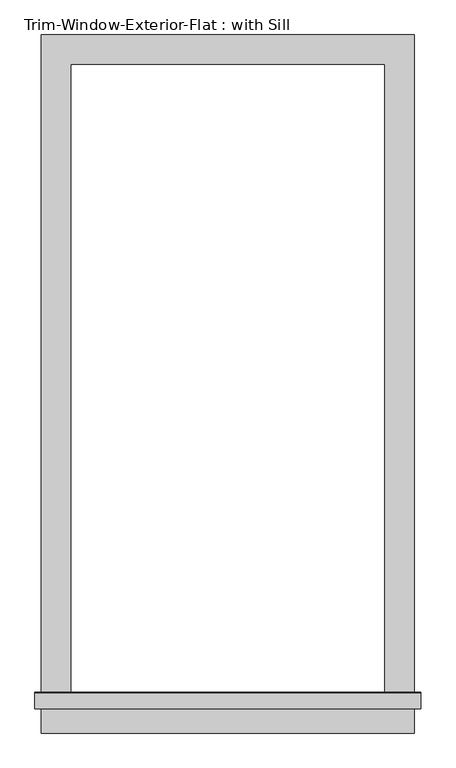
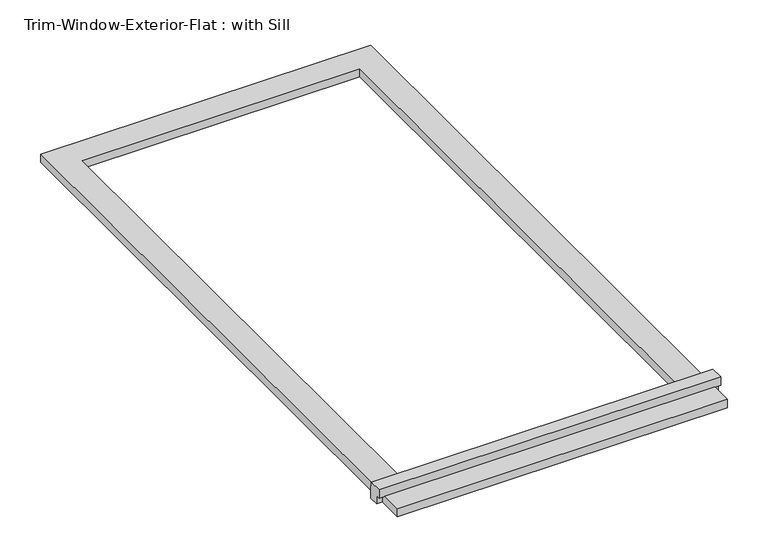
"""IFC4 building model written with IfcOpenShell, lengths in millimetres: proxy geometry, Trim-Window-Exterior-Flat : with Sill."""

from ifc_helpers import new_model, si_unit, frame, origin, origin_with_axes, place, context, project, spatial, polyline, outline, extrude, source, transform, mapped, element, save


def trim_window_exterior_flat_with_sill_35723329(model_context):
    return source(origin(), model_context, "Body", "SweptSolid", [
        extrude(outline(polyline([(361.95, -1241.3823709), (361.95, -1298.5323709), (-361.95, -1298.5323709), (-361.95, -1241.3823709), (361.95, -1241.3823709)])), origin_with_axes(), (0.0, 0.0, 1.0), 19.05),
        extrude(outline(polyline([(-1250.95, 38.1), (-1221.6580645, 38.1), (-1219.2, 19.05), (-1219.2, 0.0), (-1241.3823709, 0.0), (-1241.3823709, 19.05), (-1250.95, 19.05), (-1250.95, 38.1)])), frame((-374.65, 0.0, 0.0), z_axis=(1.0, 0.0, 0.0), x_axis=(0.0, 1.0, 0.0)), (0.0, 0.0, 1.0), 749.3),
        extrude(outline(polyline([(-361.95, 57.15), (361.95, 57.15), (361.95, -1219.2), (304.8, -1219.2), (304.8, 0.0), (-304.8, 0.0), (-304.8, -1219.2), (-361.95, -1219.2), (-361.95, 57.15)])), origin_with_axes(), (0.0, 0.0, 1.0), 19.05),
    ])


if __name__ == "__main__":
    model = new_model("IFC4")
    model_context = context("Model", 3, world=origin())
    ifc_project = project(units=[si_unit("LENGTHUNIT", "METRE", prefix="MILLI")], contexts=[model_context])
    site = spatial("IfcSite", under=ifc_project)
    building = spatial("IfcBuilding", under=site)
    placement = place(None, origin())
    trim_window_exterior_flat_with_sill_shape = trim_window_exterior_flat_with_sill_35723329(model_context)
    element("IfcBuildingElementProxy", 1, Name="Trim-Window-Exterior-Flat : with Sill", ObjectType="Trim-Window-Exterior-Flat : with Sill", at=placement, inside=building, context=model_context, shape_type="MappedRepresentation", body=[
        mapped(trim_window_exterior_flat_with_sill_shape, transform((0.0, 0.0, 0.0), x_axis=(1.0, 0.0, 0.0), y_axis=(0.0, 1.0, 0.0), z_axis=(0.0, 0.0, 1.0))),
    ])
    save(model, "model.ifc")

# Revit data of these elements
# Type "Trim-Window-Exterior-Flat : with Sill"
#   Trim Width = 0' - 2 1/4"
#   Trim Thickness_Picture Frame = 0' - 1 1/4"
#   Trim Thickness_with Sill = 0' - 0 3/4"
#   Sill Thickness = 0' - 1 1/4"
#   Opening Width [instance default] = 2' - 0"
#   Opening Height [instance default] = 3' - 0"
#   Default Elevation = 4' - 0"
#   Sill = yes
#   Picture Frame = no
#   Trim Material [instance default] = none
# Element 1 (IfcBuildingElementProxy, "Trim-Window-Exterior-Flat : with Sill")
#   Opening Height = 4' - 0"
#   Trim Material = Clad - White
#   Materials on its faces: "Clad - White"
# Materials
#   "Clad - White": class "Wood", colour RGB 242 242 238, transparency 0, Cost = 0
